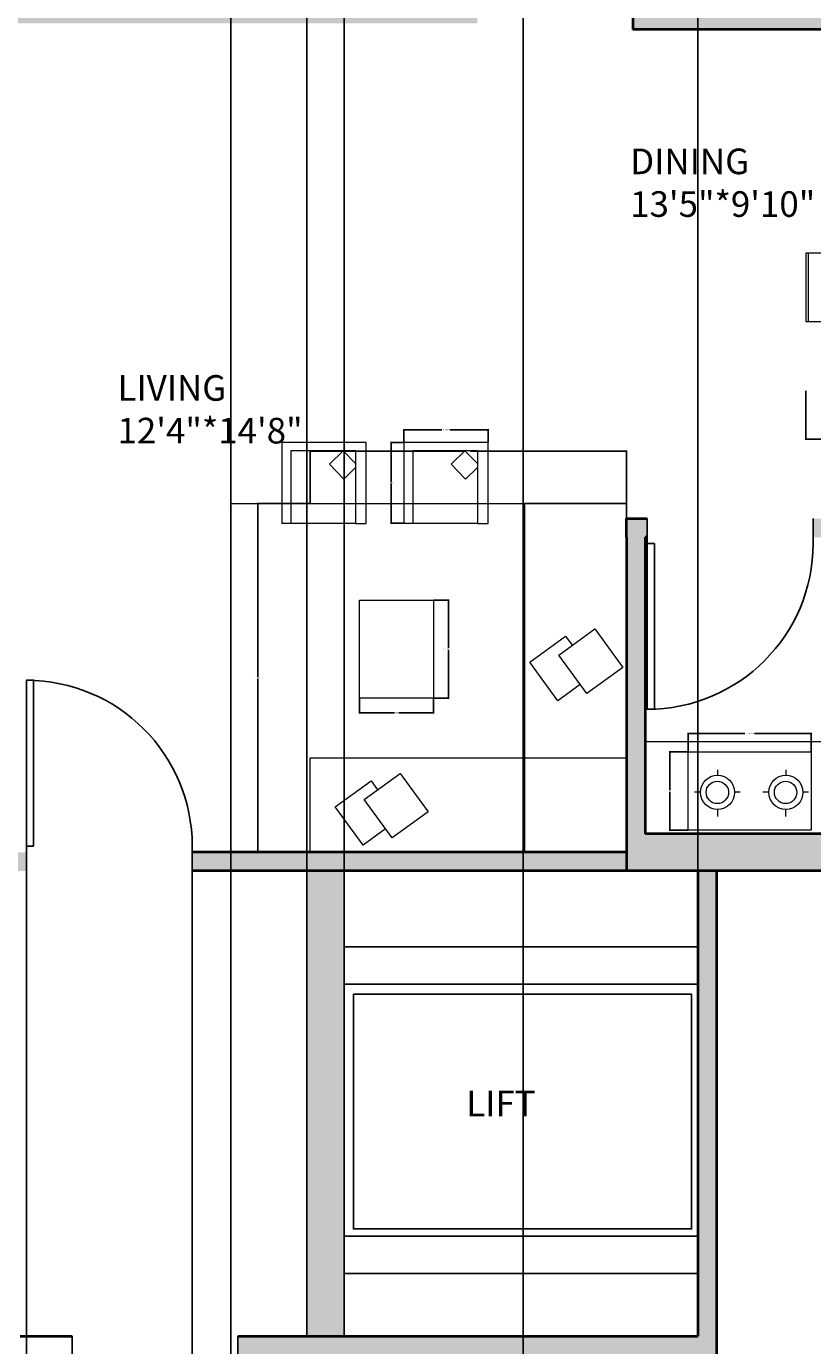
# Model space of a CAD drawing. Units: inches. Extents: x 1642 to 2399, y 1011 to 2291.
# Tile 5 of 7: x 2020 to 2210, y 1595 to 1913. Entities that reach past the tile are written whole.
import ezdxf

# ---------------------------------------------------------------- set-up
doc = ezdxf.new("R2010")
doc.units = ezdxf.units.IN
for name, color, linetype, lineweight in [('A-ANNO-DIMS', 2, 'Continuous', 18), ('A-AREA-IDEN', 7, 'Continuous', 20), ('A-DOOR', 4, 'Continuous', 25), ('A-EQPM', 8, 'Continuous', 18), ('A-FLOR-CASE', 30, 'Continuous', 18), ('A-FLOR-EVTR', 4, 'Continuous', 25), ('A-FURN', 8, 'Continuous', 18), ('A-WALL-PATT', 40, 'Continuous', 13), ('WALL', 40, 'Continuous', 40)]:
    doc.layers.add(name, color=color, linetype=linetype, lineweight=lineweight)
doc.styles.get("Standard").update_dxf_attribs({"font": 'arial.ttf'})
doc.dimstyles.get("Standard").update_dxf_attribs({"dimtxt": 0.18, "dimasz": 0.18, "dimexe": 0.18, "dimexo": 0.0625, "dimgap": 0.09, "dimtad": 0, "dimtih": 1, "dimtoh": 1, "dimdec": 4, "dimzin": 0, "dimdsep": 46, "dimtxsty": 'Standard', "dimcen": 0.09, "dimadec": 0, "dimazin": 0, "dimtfac": 1, "dimtdec": 4, "dimtofl": 0, "dimtmove": 0, "dimatfit": 3, "dimfxl": 1, "dimtolj": 1, "dimtzin": 0, "dimarcsym": 0})

# ---------------------------------------------------------------- blocks, each defined once
blk = doc.blocks.new('*U2')
for p, q in [((0, 0), (0, -6)), ((40, 0), (40, -6))]:
    blk.add_line(p, q)
blk.add_lwpolyline([(0, 0), (0, 40), (1.75, 40), (1.75, 0)], close=True)
blk.add_arc((0, 0), 40, 0, 90)
blk = doc.blocks.new('TABLE-DINING-SIX-SEAT')
for p, q in [((15.31, 48.55), (31.81, 48.55)), ((44.68, 48.55), (61.18, 48.55)), ((0.59, 16.67), (0.59, 33.17)), ((77.22, 16.83), (77.22, 33.33)), ((15.31, 0.59), (31.81, 0.59)), ((44.68, 0.59), (61.18, 0.59))]:
    blk.add_line(p, q)
for points in [[(15.31, 38.77), (31.81, 38.77), (31.81, 49.15), (15.31, 49.15)], [(44.68, 38.77), (61.18, 38.77), (61.18, 49.15), (44.68, 49.15)], [(10.38, 38.77), (67.43, 38.77), (67.43, 10.38), (10.38, 10.38)], [(10.38, 16.67), (10.38, 33.17), (0, 33.17), (0, 16.67)], [(67.43, 16.83), (67.43, 33.33), (77.81, 33.33), (77.81, 16.83)], [(15.31, 10.38), (31.81, 10.38), (31.81, 0), (15.31, 0)], [(44.68, 10.38), (61.18, 10.38), (61.18, 0), (44.68, 0)]]:
    blk.add_lwpolyline(points, close=True)
blk = doc.blocks.new('SEATING-CORNER')
for points in [[(0, 84.13), (76.26, 84.13), (76.26, 61.34), (0, 61.34)], [(0, 0), (24.56, 0), (24.56, 84.13), (0, 84.13)], [(56.51, 80.66), (63.26, 71.39), (54.61, 65.09), (47.86, 74.37)], [(9.57, 45.8), (16.32, 36.53), (7.67, 30.23), (0.92, 39.51)]]:
    blk.add_lwpolyline(points, close=True)
for points in [[(58.1, 78.48), (63.51, 82.42), (70.26, 73.15), (61.61, 66.85), (60.02, 69.03)], [(11.16, 43.62), (16.57, 47.56), (23.32, 38.28), (14.67, 31.99), (13.08, 34.17)]]:
    blk.add_lwpolyline(points)
blk = doc.blocks.new('CHAIR-LOUNGE')
for p, q in [((2.54, 19.51), (0, 19.51)), ((0, 19.51), (0, 0)), ((18.08, 19.51), (20.31, 19.51)), ((20.31, 19.32), (20.31, 19.51)), ((20.31, 0), (20.31, 19.32)), ((0, 0), (20.31, 0))]:
    blk.add_line(p, q)
blk.add_lwpolyline([(2.54, 19.51), (18.08, 19.51), (18.08, 1.93), (2.54, 1.93)], close=True)
blk.add_lwpolyline([(2.54, 6.05), (5.4, 8.82), (8.88, 5.23), (5.55, 2), (2.54, 5.1)])
blk = doc.blocks.new('COOKTOP-TWO-BURNER')
for p, q in [((6.17, 13.89), (6.17, 15.59)), ((22.64, 13.89), (22.64, 15.59)), ((2, 9.67), (0.69, 9.67)), ((10.24, 9.72), (11.69, 9.72)), ((18.47, 9.67), (17.17, 9.67)), ((26.71, 9.72), (28.17, 9.72)), ((6.02, 5.65), (6.02, 4.35)), ((22.49, 5.65), (22.49, 4.35))]:
    blk.add_line(p, q)
blk.add_lwpolyline([(0, 18.89), (29.66, 18.89), (29.66, 0), (0, 0)], close=True)
for centre, radius in [((6.12, 9.77), 4.12), ((22.59, 9.77), 4.12), ((6.17, 9.77), 2.71), ((22.64, 9.77), 2.71)]:
    blk.add_circle(centre, radius)
blk = doc.blocks.new('TABLE-COFFEE')
blk.add_lwpolyline([(0, 23.65), (17.89, 23.65), (17.89, 0), (0, 0)], close=True)
blk = doc.blocks.new('*D16')
at = {"layer": 'A-ANNO-DIMS', "color": 0, "lineweight": -2, "transparency": 16777216}
for p, q in [((2111.47, 1812.9), (2111.47, 1816.06)), ((2111.65, 1815.88), (2120.67, 1815.88)), ((2131.6, 1815.88), (2122.58, 1815.88)), ((2131.78, 1812.9), (2131.78, 1816.06))]:
    blk.add_line(p, q, dxfattribs=at)
at = {"layer": 'A-ANNO-DIMS', "color": 0, "transparency": 16777216}
for points in [[(2111.65, 1815.91), (2111.65, 1815.85), (2111.47, 1815.88)], [(2131.6, 1815.91), (2131.6, 1815.85), (2131.78, 1815.88)]]:
    blk.add_solid(points, dxfattribs=at)
at = {"layer": 'Defpoints', "color": 0, "transparency": 16777216}
for p in [(2111.47, 1815.88), (2111.47, 1812.83), (2131.78, 1812.83)]:
    blk.add_point(p, dxfattribs=at)
at = {"layer": 'A-ANNO-DIMS', "color": 0, "transparency": 16777216, "insert": (2121.63, 1815.88), "char_height": 0.18, "attachment_point": 5}
blk.add_mtext('\\A1;CHAIR 20 TYP.', dxfattribs=at)
blk = doc.blocks.new('*D17')
at = {"layer": 'A-ANNO-DIMS', "color": 0, "lineweight": -2, "transparency": 16777216}
for p, q in [((2111.41, 1812.83), (2108.25, 1812.83)), ((2108.43, 1812.65), (2108.43, 1803.26)), ((2108.43, 1793.51), (2108.43, 1802.9)), ((2111.41, 1793.33), (2108.25, 1793.33))]:
    blk.add_line(p, q, dxfattribs=at)
at = {"layer": 'A-ANNO-DIMS', "color": 0, "transparency": 16777216}
for points in [[(2108.4, 1812.65), (2108.46, 1812.65), (2108.43, 1812.83)], [(2108.4, 1793.51), (2108.46, 1793.51), (2108.43, 1793.33)]]:
    blk.add_solid(points, dxfattribs=at)
at = {"layer": 'Defpoints', "color": 0, "transparency": 16777216}
for p in [(2111.47, 1812.83), (2108.43, 1793.33), (2111.47, 1793.33)]:
    blk.add_point(p, dxfattribs=at)
at = {"layer": 'A-ANNO-DIMS', "color": 0, "transparency": 16777216, "insert": (2108.43, 1803.08), "char_height": 0.18, "attachment_point": 5}
blk.add_mtext('\\A1;20 TYP.', dxfattribs=at)
blk = doc.blocks.new('*D18')
at = {"layer": 'A-ANNO-DIMS', "color": 0, "lineweight": -2, "transparency": 16777216}
for p, q in [((2208.46, 1825.25), (2208.46, 1813.46)), ((2286.28, 1825.25), (2286.28, 1813.46)), ((2208.64, 1813.64), (2246.09, 1813.64)), ((2286.1, 1813.64), (2248.65, 1813.64))]:
    blk.add_line(p, q, dxfattribs=at)
at = {"layer": 'A-ANNO-DIMS', "color": 0, "transparency": 16777216}
for points in [[(2208.64, 1813.67), (2208.64, 1813.61), (2208.46, 1813.64)], [(2286.1, 1813.67), (2286.1, 1813.61), (2286.28, 1813.64)]]:
    blk.add_solid(points, dxfattribs=at)
at = {"layer": 'Defpoints', "color": 0, "transparency": 16777216}
for p in [(2208.46, 1825.31), (2286.28, 1825.31), (2286.28, 1813.64)]:
    blk.add_point(p, dxfattribs=at)
at = {"layer": 'A-ANNO-DIMS', "color": 0, "transparency": 16777216, "insert": (2247.37, 1813.64), "char_height": 0.18, "attachment_point": 5}
blk.add_mtext('\\A1;DINING SET 78 TYP.', dxfattribs=at)
blk = doc.blocks.new('*D20')
at = {"layer": 'A-ANNO-DIMS', "color": 0, "lineweight": -2, "transparency": 16777216}
for p, q in [((2088.86, 1798.08), (2076.12, 1798.08)), ((2076.3, 1797.9), (2076.3, 1756.2)), ((2076.3, 1714.14), (2076.3, 1755.84)), ((2088.86, 1713.96), (2076.12, 1713.96))]:
    blk.add_line(p, q, dxfattribs=at)
at = {"layer": 'A-ANNO-DIMS', "color": 0, "transparency": 16777216}
for points in [[(2076.27, 1797.9), (2076.33, 1797.9), (2076.3, 1798.08)], [(2076.27, 1714.14), (2076.33, 1714.14), (2076.3, 1713.96)]]:
    blk.add_solid(points, dxfattribs=at)
at = {"layer": 'Defpoints', "color": 0, "transparency": 16777216}
for p in [(2088.92, 1798.08), (2076.3, 1713.96), (2088.92, 1713.96)]:
    blk.add_point(p, dxfattribs=at)
at = {"layer": 'A-ANNO-DIMS', "color": 0, "transparency": 16777216, "insert": (2076.3, 1756.02), "char_height": 0.18, "attachment_point": 5}
blk.add_mtext('\\A1;CORNER SOFA 84 TYP.', dxfattribs=at)
blk = doc.blocks.new('*D21')
at = {"layer": 'A-ANNO-DIMS', "color": 0, "lineweight": -2, "transparency": 16777216}
for p, q in [((2088.92, 1798.15), (2088.92, 1810.88)), ((2165.18, 1798.15), (2165.18, 1810.88)), ((2089.1, 1810.7), (2126.52, 1810.7)), ((2165, 1810.7), (2127.58, 1810.7))]:
    blk.add_line(p, q, dxfattribs=at)
at = {"layer": 'A-ANNO-DIMS', "color": 0, "transparency": 16777216}
for points in [[(2089.1, 1810.73), (2089.1, 1810.67), (2088.92, 1810.7)], [(2165, 1810.73), (2165, 1810.67), (2165.18, 1810.7)]]:
    blk.add_solid(points, dxfattribs=at)
at = {"layer": 'Defpoints', "color": 0, "transparency": 16777216}
for p in [(2088.92, 1810.7), (2088.92, 1798.08), (2165.18, 1798.08)]:
    blk.add_point(p, dxfattribs=at)
at = {"layer": 'A-ANNO-DIMS', "color": 0, "transparency": 16777216, "insert": (2127.05, 1810.7), "char_height": 0.18, "attachment_point": 5}
blk.add_mtext('\\A1;76 TYP.', dxfattribs=at)
blk = doc.blocks.new('*D22')
at = {"layer": 'A-ANNO-DIMS', "color": 0, "lineweight": -2, "transparency": 16777216}
for p, q in [((2180.07, 1738.26), (2180.07, 1742.82)), ((2180.25, 1742.64), (2193.71, 1742.64)), ((2209.55, 1742.64), (2196.09, 1742.64)), ((2209.73, 1738.26), (2209.73, 1742.82))]:
    blk.add_line(p, q, dxfattribs=at)
at = {"layer": 'A-ANNO-DIMS', "color": 0, "transparency": 16777216}
for points in [[(2180.25, 1742.67), (2180.25, 1742.61), (2180.07, 1742.64)], [(2209.55, 1742.67), (2209.55, 1742.61), (2209.73, 1742.64)]]:
    blk.add_solid(points, dxfattribs=at)
at = {"layer": 'Defpoints', "color": 0, "transparency": 16777216}
for p in [(2180.07, 1742.64), (2180.07, 1738.19), (2209.73, 1738.19)]:
    blk.add_point(p, dxfattribs=at)
at = {"layer": 'A-ANNO-DIMS', "color": 0, "transparency": 16777216, "insert": (2194.9, 1742.64), "char_height": 0.18, "attachment_point": 5}
blk.add_mtext('\\A1;COOKTOP 30 TYP.', dxfattribs=at)
blk = doc.blocks.new('*D23')
at = {"layer": 'A-ANNO-DIMS', "color": 0, "lineweight": -2, "transparency": 16777216}
for p, q in [((2180.01, 1738.19), (2175.44, 1738.19)), ((2175.62, 1738.01), (2175.62, 1728.93)), ((2175.62, 1719.49), (2175.62, 1728.57)), ((2180.01, 1719.31), (2175.44, 1719.31))]:
    blk.add_line(p, q, dxfattribs=at)
at = {"layer": 'A-ANNO-DIMS', "color": 0, "transparency": 16777216}
for points in [[(2175.59, 1738.01), (2175.65, 1738.01), (2175.62, 1738.19)], [(2175.59, 1719.49), (2175.65, 1719.49), (2175.62, 1719.31)]]:
    blk.add_solid(points, dxfattribs=at)
at = {"layer": 'Defpoints', "color": 0, "transparency": 16777216}
for p in [(2180.07, 1738.19), (2175.62, 1719.31), (2180.07, 1719.31)]:
    blk.add_point(p, dxfattribs=at)
at = {"layer": 'A-ANNO-DIMS', "color": 0, "transparency": 16777216, "insert": (2175.62, 1728.75), "char_height": 0.18, "attachment_point": 5}
blk.add_mtext('\\A1;19 TYP.', dxfattribs=at)
blk = doc.blocks.new('*D28')
at = {"layer": 'A-ANNO-DIMS', "color": 0, "lineweight": -2, "transparency": 16777216}
for p, q in [((2118.74, 1774.81), (2122.4, 1774.81)), ((2122.22, 1774.63), (2122.22, 1763.17)), ((2122.22, 1751.34), (2122.22, 1762.8)), ((2118.74, 1751.16), (2122.4, 1751.16))]:
    blk.add_line(p, q, dxfattribs=at)
at = {"layer": 'A-ANNO-DIMS', "color": 0, "transparency": 16777216}
for points in [[(2122.19, 1774.63), (2122.25, 1774.63), (2122.22, 1774.81)], [(2122.19, 1751.34), (2122.25, 1751.34), (2122.22, 1751.16)]]:
    blk.add_solid(points, dxfattribs=at)
at = {"layer": 'Defpoints', "color": 0, "transparency": 16777216}
for p in [(2118.67, 1774.81), (2118.67, 1751.16), (2122.22, 1751.16)]:
    blk.add_point(p, dxfattribs=at)
at = {"layer": 'A-ANNO-DIMS', "color": 0, "transparency": 16777216, "insert": (2122.22, 1762.99), "char_height": 0.18, "attachment_point": 5}
blk.add_mtext('\\A1;COFFEE TABLE 24 TYP.', dxfattribs=at)
blk = doc.blocks.new('*D29')
at = {"layer": 'A-ANNO-DIMS', "color": 0, "lineweight": -2, "transparency": 16777216}
for p, q in [((2100.78, 1751.1), (2100.78, 1747.43)), ((2118.67, 1751.1), (2118.67, 1747.43)), ((2100.96, 1747.61), (2109.21, 1747.61)), ((2118.49, 1747.61), (2110.25, 1747.61))]:
    blk.add_line(p, q, dxfattribs=at)
at = {"layer": 'A-ANNO-DIMS', "color": 0, "transparency": 16777216}
for points in [[(2100.96, 1747.64), (2100.96, 1747.58), (2100.78, 1747.61)], [(2118.49, 1747.64), (2118.49, 1747.58), (2118.67, 1747.61)]]:
    blk.add_solid(points, dxfattribs=at)
at = {"layer": 'Defpoints', "color": 0, "transparency": 16777216}
for p in [(2100.78, 1751.16), (2118.67, 1751.16), (2100.78, 1747.61)]:
    blk.add_point(p, dxfattribs=at)
at = {"layer": 'A-ANNO-DIMS', "color": 0, "transparency": 16777216, "insert": (2109.73, 1747.61), "char_height": 0.18, "attachment_point": 5}
blk.add_mtext('\\A1;18 TYP.', dxfattribs=at)
blk = doc.blocks.new('*D40')
at = {"layer": 'A-ANNO-DIMS', "color": 0, "lineweight": -2, "transparency": 16777216}
for p, q in [((1796.18, 1709.39), (1796.18, 1011.19)), ((2186.88, 1709.39), (2186.88, 1011.19)), ((1796.36, 1011.37), (1991.13, 1011.37)), ((2186.7, 1011.37), (1991.92, 1011.37))]:
    blk.add_line(p, q, dxfattribs=at)
at = {"layer": 'A-ANNO-DIMS', "color": 0, "transparency": 16777216}
for points in [[(1796.36, 1011.4), (1796.36, 1011.34), (1796.18, 1011.37)], [(2186.7, 1011.4), (2186.7, 1011.34), (2186.88, 1011.37)]]:
    blk.add_solid(points, dxfattribs=at)
at = {"layer": 'Defpoints', "color": 0, "transparency": 16777216}
for p in [(1796.18, 1709.46), (2186.88, 1709.46), (2186.88, 1011.37)]:
    blk.add_point(p, dxfattribs=at)
at = {"layer": 'A-ANNO-DIMS', "color": 0, "transparency": 16777216, "insert": (1991.53, 1011.37), "char_height": 0.18, "attachment_point": 5}
blk.add_mtext('\\A1;390.7', dxfattribs=at)
blk = doc.blocks.new('*D42')
at = {"layer": 'A-ANNO-DIMS', "color": 0, "lineweight": -2, "transparency": 16777216}
for p, q in [((1946.68, 1597.27), (1946.68, 2290.98)), ((1946.86, 2290.8), (2016.99, 2290.8)), ((2087.89, 2290.8), (2017.76, 2290.8)), ((2088.07, 1597.27), (2088.07, 2290.98))]:
    blk.add_line(p, q, dxfattribs=at)
at = {"layer": 'A-ANNO-DIMS', "color": 0, "transparency": 16777216}
for points in [[(1946.86, 2290.83), (1946.86, 2290.77), (1946.68, 2290.8)], [(2087.89, 2290.83), (2087.89, 2290.77), (2088.07, 2290.8)]]:
    blk.add_solid(points, dxfattribs=at)
at = {"layer": 'Defpoints', "color": 0, "transparency": 16777216}
for p in [(2088.07, 2290.8), (1946.68, 1597.21), (2088.07, 1597.21)]:
    blk.add_point(p, dxfattribs=at)
at = {"layer": 'A-ANNO-DIMS', "color": 0, "transparency": 16777216, "insert": (2017.37, 2290.8), "char_height": 0.18, "attachment_point": 5}
blk.add_mtext('\\A1;141.4', dxfattribs=at)
blk = doc.blocks.new('*D43')
at = {"layer": 'A-ANNO-DIMS', "color": 0, "lineweight": -2, "transparency": 16777216}
for p, q in [((2097.07, 1597.27), (2097.07, 2290.98)), ((2097.25, 2290.8), (2139.35, 2290.8)), ((2182.2, 2290.8), (2140.1, 2290.8)), ((2182.38, 1597.27), (2182.38, 2290.98))]:
    blk.add_line(p, q, dxfattribs=at)
at = {"layer": 'A-ANNO-DIMS', "color": 0, "transparency": 16777216}
for points in [[(2097.25, 2290.83), (2097.25, 2290.77), (2097.07, 2290.8)], [(2182.2, 2290.83), (2182.2, 2290.77), (2182.38, 2290.8)]]:
    blk.add_solid(points, dxfattribs=at)
at = {"layer": 'Defpoints', "color": 0, "transparency": 16777216}
for p in [(2182.38, 2290.8), (2097.07, 1597.21), (2182.38, 1597.21)]:
    blk.add_point(p, dxfattribs=at)
at = {"layer": 'A-ANNO-DIMS', "color": 0, "transparency": 16777216, "insert": (2139.72, 2290.8), "char_height": 0.18, "attachment_point": 5}
blk.add_mtext('\\A1;85.31', dxfattribs=at)
blk = doc.blocks.new('*D46')
at = {"layer": 'A-ANNO-DIMS', "color": 0, "lineweight": -2, "transparency": 16777216}
for p, q in [((2020.45, 1709.39), (2020.45, 1011.19)), ((2060.45, 1709.39), (2060.45, 1011.19)), ((2020.63, 1011.37), (2040.22, 1011.37)), ((2060.27, 1011.37), (2040.67, 1011.37))]:
    blk.add_line(p, q, dxfattribs=at)
at = {"layer": 'A-ANNO-DIMS', "color": 0, "transparency": 16777216}
for points in [[(2020.63, 1011.4), (2020.63, 1011.34), (2020.45, 1011.37)], [(2060.27, 1011.4), (2060.27, 1011.34), (2060.45, 1011.37)]]:
    blk.add_solid(points, dxfattribs=at)
at = {"layer": 'Defpoints', "color": 0, "transparency": 16777216}
for p in [(2020.45, 1709.46), (2060.45, 1709.46), (2060.45, 1011.37)]:
    blk.add_point(p, dxfattribs=at)
at = {"layer": 'A-ANNO-DIMS', "color": 0, "transparency": 16777216, "insert": (2040.45, 1011.37), "char_height": 0.18, "attachment_point": 5}
blk.add_mtext('\\A1;40', dxfattribs=at)
blk = doc.blocks.new('*D48')
at = {"layer": 'A-ANNO-DIMS', "color": 0, "lineweight": -2, "transparency": 16777216}
for p, q in [((1922.74, 1392.77), (1922.74, 2290.98)), ((1922.92, 2290.8), (2031.1, 2290.8)), ((2140.06, 2290.8), (2031.89, 2290.8)), ((2140.24, 1392.77), (2140.24, 2290.98))]:
    blk.add_line(p, q, dxfattribs=at)
at = {"layer": 'A-ANNO-DIMS', "color": 0, "transparency": 16777216}
for points in [[(1922.92, 2290.83), (1922.92, 2290.77), (1922.74, 2290.8)], [(2140.06, 2290.83), (2140.06, 2290.77), (2140.24, 2290.8)]]:
    blk.add_solid(points, dxfattribs=at)
at = {"layer": 'Defpoints', "color": 0, "transparency": 16777216}
for p in [(2140.24, 2290.8), (1922.74, 1392.71), (2140.24, 1392.71)]:
    blk.add_point(p, dxfattribs=at)
at = {"layer": 'A-ANNO-DIMS', "color": 0, "transparency": 16777216, "insert": (2031.49, 2290.8), "char_height": 0.18, "attachment_point": 5}
blk.add_mtext('\\A1;217.5', dxfattribs=at)
blk = doc.blocks.new('*D50')
at = {"layer": 'A-ANNO-DIMS', "color": 0, "lineweight": -2, "transparency": 16777216}
for p, q in [((1993.24, 1295.77), (1993.24, 2290.98)), ((1993.42, 2290.8), (2031.17, 2290.8)), ((2069.56, 2290.8), (2031.82, 2290.8)), ((2069.74, 1295.77), (2069.74, 2290.98))]:
    blk.add_line(p, q, dxfattribs=at)
at = {"layer": 'A-ANNO-DIMS', "color": 0, "transparency": 16777216}
for points in [[(1993.42, 2290.83), (1993.42, 2290.77), (1993.24, 2290.8)], [(2069.56, 2290.83), (2069.56, 2290.77), (2069.74, 2290.8)]]:
    blk.add_solid(points, dxfattribs=at)
at = {"layer": 'Defpoints', "color": 0, "transparency": 16777216}
for p in [(2069.74, 2290.8), (1993.24, 1295.71), (2069.74, 1295.71)]:
    blk.add_point(p, dxfattribs=at)
at = {"layer": 'A-ANNO-DIMS', "color": 0, "transparency": 16777216, "insert": (2031.49, 2290.8), "char_height": 0.18, "attachment_point": 5}
blk.add_mtext('\\A1;76.5', dxfattribs=at)

msp = doc.modelspace()

# ---------------------------------------------------------------- hatches: boundary and pattern name
at = {"layer": 'A-WALL-PATT'}
h = msp.add_hatch(color=256, dxfattribs=at)
h.dxf.hatch_style = 1
h.paths.add_polyline_path([(2340.1804, 2185.4562), (2211.0983, 2185.4562, -0.01876983), (2211.211, 2182.4562), (2211.211, 2176.4562), (2331.211, 2176.4562), (2331.211, 2043.4562), (2171.211, 2043.4562), (2171.211, 2038.9562), (2331.211, 2038.9562), (2331.211, 1916.9562), (2171.211, 1916.9562), (2171.211, 1918.9365), (2166.711, 1918.9365), (2166.711, 1912.4562), (2340.1804, 1912.4562)])
h.paths.add_polyline_path([(2171.211, 2043.4562), (2171.211, 2043.9025), (2170.5217, 2043.9025), (2166.711, 2043.9025), (2166.711, 2038.9562), (2166.711, 1958.9365), (2171.211, 1958.9365)], flags=17)
h.paths.add_polyline_path([(2129.211, 1971.5979), (2124.711, 1971.5979), (2124.711, 1918.4562), (2067.711, 1918.4562), (2067.711, 1913.9562), (2129.211, 1913.9562)])
h.paths.add_polyline_path([(2067.711, 2015.4562), (2124.711, 2015.4562), (2124.711, 2019.9562), (2058.711, 2019.9562), (2058.711, 2015.4562), (2058.711, 1922.9562), (1982.211, 1922.9562), (1982.211, 2015.4562), (1982.211, 2019.9562), (1916.211, 2019.9562), (1916.211, 2070.9562), (1911.711, 2070.9562), (1911.711, 2015.4562), (1911.711, 2012.302), (1916.211, 2012.302), (1916.211, 2015.4562), (1973.211, 2015.4562), (1973.211, 1918.4562), (1973.211, 1913.9562), (2017.1804, 1913.9562), (2067.711, 1913.9562), (2067.711, 1918.4562)])
h.paths.add_polyline_path([(2131.1386, 2075.4562), (2118.1934, 2075.4562), (2118.1934, 2070.9562), (2131.1386, 2070.9562)], flags=17)
h.paths.add_polyline_path([(1918.8034, 2075.4562), (1909.4956, 2075.4562), (1909.4956, 2070.9562), (1918.8034, 2070.9562)], flags=17)
h.paths.add_polyline_path([(1874.211, 2029.9562), (1869.711, 2029.9562), (1869.711, 1960.7404), (1874.211, 1960.7404)], flags=17)
h.paths.add_polyline_path([(1916.211, 1972.302), (1911.711, 1972.302), (1911.711, 1918.4562), (1916.211, 1918.4562)], flags=17)
h.paths.add_polyline_path([(2340.1804, 1912.4562), (2331.1804, 1912.4562), (2331.1804, 1794.4562), (2210.1804, 1794.4562), (2210.1804, 1789.9562), (2279.6804, 1789.9562), (2340.1804, 1789.9562)])
h.paths.add_polyline_path([(2288.6804, 1789.9562), (2279.6804, 1789.9562), (2279.6804, 1785.0846), (2285.6804, 1785.0846), (2288.6804, 1785.0846)], flags=17)
h.paths.add_polyline_path([(2169.6804, 1789.9562), (2170.1804, 1789.9562), (2170.1804, 1794.4562), (2165.1804, 1794.4562), (2165.1804, 1713.9562), (2165.1804, 1709.4562), (2279.6804, 1709.4562), (2279.6804, 1718.4562), (2169.6804, 1718.4562)])
h.paths.add_polyline_path([(2288.6804, 1745.1973, -0.01876983), (2285.6804, 1745.0846), (2279.6804, 1745.0846), (2279.6804, 1709.4562), (2340.1804, 1709.4562), (2340.1804, 1789.9562), (2335.6804, 1789.9562), (2335.6804, 1713.9562), (2288.6804, 1713.9562)])
h.paths.add_polyline_path([(2165.1804, 1713.9562), (2140.6229, 1713.9562), (2088.923, 1713.9562), (2069.7509, 1713.9562), (2060.4457, 1713.9562), (2060.4457, 1709.4562), (2165.1804, 1709.4562)])
h.paths.add_polyline_path([(2020.4457, 1713.9562), (2017.1804, 1713.9562), (2012.6804, 1713.9562), (2009.1946, 1713.9562), (2009.1946, 1709.4562), (2020.4457, 1709.4562)])
h.paths.add_polyline_path([(1969.1946, 1713.9562), (1864.6804, 1713.9562), (1864.6804, 1798.9562), (1860.1804, 1798.9562), (1860.1804, 1792.9562), (1860.1804, 1752.9562), (1860.1804, 1718.4562), (1750.1804, 1718.4562), (1750.1804, 1749.2419), (1744.1804, 1749.2419, -0.01876983), (1741.1804, 1749.3546), (1741.1804, 1709.4562), (1969.1946, 1709.4562)])
h.paths.add_polyline_path([(1741.1804, 1803.4562), (1700.711, 1803.4562), (1700.711, 1794.4562), (1741.1804, 1794.4562)])
h.paths.add_polyline_path([(1820.1804, 1798.9562), (1741.1804, 1798.9562), (1741.1804, 1794.4562), (1741.1804, 1790.0365), (1741.1804, 1789.2419), (1744.1804, 1789.2419), (1750.1804, 1789.2419), (1750.1804, 1794.4562), (1820.1804, 1794.4562)], flags=17)
h.paths.add_polyline_path([(1800.6804, 1709.4562), (1796.1804, 1709.4562), (1796.1804, 1592.7078), (1978.9325, 1592.7078), (1978.9325, 1597.2078), (1800.6804, 1597.2078)])
h.paths.add_polyline_path([(2097.0678, 1709.4562), (2088.0678, 1709.4562), (2088.0678, 1599.6874), (2088.0678, 1597.2078), (2097.0678, 1597.2078)], flags=17)
h.paths.add_polyline_path([(2186.8766, 1709.4562), (2182.3766, 1709.4562), (2182.3766, 1597.2078), (2071.4624, 1597.2078), (2071.4624, 1592.7078), (2186.8766, 1592.7078)])
h.paths.add_polyline_path([(2078.1934, 2075.4562), (2022.711, 2075.4562), (2022.711, 2223.4562), (2166.711, 2223.4562), (2166.711, 2075.4562), (2166.711, 2070.9562), (2171.211, 2070.9562), (2171.211, 2138.8919), (2171.211, 2227.9562), (2335.711, 2227.9562), (2335.711, 2185.4562), (2340.1804, 2185.4562), (2340.1804, 2232.4562), (1874.211, 2232.4562), (1874.211, 2223.4562), (2018.211, 2223.4562), (2018.211, 2075.4562), (1958.8034, 2075.4562), (1958.8034, 2070.9562), (2018.211, 2070.9562), (2018.211, 2019.9562), (1982.211, 2019.9562), (1982.211, 2015.4562), (1982.211, 2010.9562), (2058.711, 2010.9562), (2058.711, 2015.4562), (2058.711, 2019.9562), (2022.711, 2019.9562), (2022.711, 2070.9562), (2078.1934, 2070.9562)])
h.paths.add_polyline_path([(1874.211, 2171.9562), (1874.211, 2176.4562), (1861.9371, 2176.4562), (1861.9371, 2173.4562), (1861.9371, 2167.4562), (1869.711, 2167.4562), (1869.711, 2069.7602), (1874.211, 2069.7602)], flags=17)
h.paths.add_polyline_path([(1705.211, 2227.9562), (1865.211, 2227.9562), (1865.211, 2176.4562), (1874.211, 2176.4562), (1874.211, 2232.4562), (1700.711, 2232.4562), (1700.711, 2176.4562), (1705.211, 2176.4562)])
h.paths.add_polyline_path([(1709.711, 2167.4562), (1821.9371, 2167.4562), (1821.9371, 2173.4562, -0.01876983), (1822.0498, 2176.4562), (1700.711, 2176.4562), (1700.711, 1913.9562), (1860.1804, 1913.9562), (1864.6804, 1913.9562), (1973.211, 1913.9562), (1973.211, 1918.4562), (1916.211, 1918.4562), (1874.211, 1918.4562), (1874.211, 1920.7404), (1869.711, 1920.7404), (1869.711, 1918.4562), (1860.1804, 1918.4562), (1709.711, 1918.4562), (1709.711, 2029.9562), (1874.211, 2029.9562), (1874.211, 2037.0364), (1869.711, 2037.0364), (1869.711, 2034.4562), (1709.711, 2034.4562)])
h.paths.add_polyline_path([(2017.1804, 1913.9562), (2012.6804, 1913.9562), (2012.6804, 1713.9562), (2017.1804, 1713.9562)])
h.paths.add_polyline_path([(1952.4341, 2110.3716), (2000.4134, 2110.3716), (2000.4134, 2133.4189), (1952.4341, 2133.4189)], flags=25)
h.paths.add_polyline_path([(2042.3983, 2110.7121), (2090.3775, 2110.7121), (2090.3775, 2133.7594), (2042.3983, 2133.7594)], flags=25)
h.paths.add_polyline_path([(2201.7332, 2091.8715), (2249.7125, 2091.8715), (2249.7125, 2114.9188), (2201.7332, 2114.9188)], flags=25)
h.paths.add_polyline_path([(1805.186, 2077.6915), (1853.1653, 2077.6915), (1853.1653, 2100.7388), (1805.186, 2100.7388)], flags=25)
h.paths.add_polyline_path([(1794.8897, 1974.6584), (1842.869, 1974.6584), (1842.869, 1997.7057), (1794.8897, 1997.7057)], flags=25)
h.paths.add_polyline_path([(2229.1796, 2204.4209), (2315.1362, 2204.4209), (2315.1362, 2217.1488), (2229.1796, 2217.1488)], flags=25)
h.paths.add_polyline_path([(1715.2159, 2199.5328), (1801.1724, 2199.5328), (1801.1724, 2212.2607), (1715.2159, 2212.2607)], flags=25)
h.paths.add_polyline_path([(2230.7681, 1755.7109), (2271.7283, 1755.7109), (2271.7283, 1778.7582), (2230.7681, 1778.7582)], flags=25)
h.paths.add_polyline_path([(1763.4713, 1764.1742), (1804.4315, 1764.1742), (1804.4315, 1787.2215), (1763.4713, 1787.2215)], flags=25)
h.paths.add_polyline_path([(2076.2643, 1955.0495), (2111.326, 1955.0495), (2111.326, 1978.0968), (2076.2643, 1978.0968)], flags=25)
h.paths.add_polyline_path([(1932.854, 1956.1217), (1967.9158, 1956.1217), (1967.9158, 1979.169), (1932.854, 1979.169)], flags=25)
h.paths.add_polyline_path([(2048.1203, 2031.6107), (2083.1821, 2031.6107), (2083.1821, 2054.658), (2048.1203, 2054.658)], flags=25)
h.paths.add_polyline_path([(2163.5754, 1863.7569), (2208.2347, 1863.7569), (2208.2347, 1886.8042), (2163.5754, 1886.8042)], flags=9)
h.paths.add_polyline_path([(2039.9286, 1809.0957), (2084.5879, 1809.0957), (2084.5879, 1832.143), (2039.9286, 1832.143)], flags=9)
h.paths.add_polyline_path([(1901.0045, 1814.0452), (1945.6638, 1814.0452), (1945.6638, 1837.0925), (1901.0045, 1837.0925)], flags=9)
h.paths.add_polyline_path([(1833.7282, 1852.5627), (1878.3875, 1852.5627), (1878.3875, 1875.61), (1833.7282, 1875.61)], flags=9)
h.paths.add_polyline_path([(2219.1375, 1926.2139), (2267.1167, 1926.2139), (2267.1167, 1949.2612), (2219.1375, 1949.2612)], flags=25)
h.paths.add_polyline_path([(1956.9598, 2029.7735), (1992.0216, 2029.7735), (1992.0216, 2052.8208), (1956.9598, 2052.8208)], flags=25)
h.paths.add_polyline_path([(2229.3, 1523.3399), (2270.2602, 1523.3399), (2270.2602, 1546.3872), (2229.3, 1546.3872)], flags=9)
h.paths.add_polyline_path([(1772.3039, 1526.9922), (1813.2641, 1526.9922), (1813.2641, 1550.0394), (1772.3039, 1550.0394)], flags=9)
h.paths.add_polyline_path([(2172.587, 1420.6999), (2217.2463, 1420.6999), (2217.2463, 1443.7472), (2172.587, 1443.7472)], flags=9)
h.paths.add_polyline_path([(1814.3549, 1422.215), (1859.0143, 1422.215), (1859.0143, 1445.2623), (1814.3549, 1445.2623)], flags=9)
h.paths.add_polyline_path([(2186.0372, 1305.6227), (2234.0165, 1305.6227), (2234.0165, 1328.67), (2186.0372, 1328.67)], flags=9)
h.paths.add_polyline_path([(1756.747, 1349.0694), (1804.7263, 1349.0694), (1804.7263, 1372.1167), (1756.747, 1372.1167)], flags=9)
h.paths.add_polyline_path([(2239.449, 1214.6184), (2287.4282, 1214.6184), (2287.4282, 1237.6657), (2239.449, 1237.6657)], flags=9)
h.paths.add_polyline_path([(1767.104, 1213.8348), (1815.0832, 1213.8348), (1815.0832, 1236.8821), (1767.104, 1236.8821)], flags=9)
h.paths.add_polyline_path([(2046.6809, 1183.6854), (2094.6602, 1183.6854), (2094.6602, 1206.7327), (2046.6809, 1206.7327)], flags=9)
h.paths.add_polyline_path([(1947.2155, 1183.6854), (1995.1948, 1183.6854), (1995.1948, 1206.7327), (1947.2155, 1206.7327)], flags=9)
h.paths.add_polyline_path([(1959.3556, 1258.7871), (1994.4174, 1258.7871), (1994.4174, 1281.8344), (1959.3556, 1281.8344)], flags=9)
h.paths.add_polyline_path([(2049.6419, 1248.9629), (2084.7036, 1248.9629), (2084.7036, 1272.0102), (2049.6419, 1272.0102)], flags=9)
h.paths.add_polyline_path([(2092.7532, 1327.4852), (2127.815, 1327.4852), (2127.815, 1350.5325), (2092.7532, 1350.5325)], flags=9)
h.paths.add_polyline_path([(1944.9358, 1327.4852), (1979.9976, 1327.4852), (1979.9976, 1350.5325), (1944.9358, 1350.5325)], flags=9)
h.paths.add_polyline_path([(1974.5055, 1650.063), (2006.3695, 1650.063), (2006.3695, 1662.7909), (1974.5055, 1662.7909)], flags=9)

# ---------------------------------------------------------------- linework, layer by layer
at = {"layer": 'A-FLOR-CASE'}
msp.add_line((2279.6804, 1740.5928), (2169.6804, 1740.5928), dxfattribs=at)
at = {"layer": 'A-FLOR-EVTR'}
for p, q in [((2088.0678, 1599.6874), (2088.0678, 1711.9358)), ((2088.0678, 1597.2078), (2088.0678, 1709.4562)), ((2097.0678, 1597.2078), (2097.0678, 1709.4562)), ((2097.0678, 1691.1483), (2182.3766, 1691.1483)), ((2097.0678, 1682.1483), (2182.3766, 1682.1483)), ((2097.0678, 1621.3756), (2182.3766, 1621.3756)), ((2097.0678, 1612.3756), (2182.3766, 1612.3756))]:
    msp.add_line(p, q, dxfattribs=at)
msp.add_lwpolyline([(2099.3395, 1679.7065), (2180.8762, 1679.7065), (2180.8762, 1623.0927), (2099.3395, 1623.0927)], close=True, dxfattribs=at)
at = {"layer": 'A-FURN'}
msp.add_lwpolyline([(2165.1804, 1713.9562), (2069.7509, 1713.9562), (2069.7509, 1798.0844), (2165.1804, 1798.0844)], close=True, dxfattribs=at)
at = {"layer": 'WALL'}
for p, q in [((2166.711, 1918.9365), (2166.711, 1912.4562)), ((2340.211, 1912.4562), (2166.711, 1912.4562)), ((2165.1804, 1789.9562), (2165.1804, 1794.4562)), ((2165.1804, 1794.4562), (2170.1804, 1794.4562)), ((2165.1804, 1789.9562), (2165.1804, 1709.4562)), ((2169.6804, 1789.9562), (2169.6804, 1718.4562)), ((2170.1804, 1789.9562), (2169.6804, 1789.9562)), ((2279.6804, 1718.4562), (2169.6804, 1718.4562)), ((2165.1804, 1713.9562), (2060.4457, 1713.9562)), ((2165.1804, 1713.9562), (2060.4457, 1713.9562)), ((2165.1804, 1709.4562), (2060.4457, 1709.4562)), ((2279.6804, 1709.4562), (2165.1804, 1709.4562)), ((2182.3766, 1709.4562), (2182.3766, 1597.2078)), ((2186.8766, 1709.4562), (2186.8766, 1592.7078)), ((2018.9325, 1597.2078), (2031.4624, 1597.2078)), ((2071.4624, 1597.2078), (2182.3766, 1597.2078))]:
    msp.add_line(p, q, dxfattribs=at)
msp.add_lwpolyline([(1969.1946, 1709.4562), (1700.711, 1709.4562), (1700.711, 2232.4562), (2340.1804, 2232.4562), (2340.1804, 1709.4562), (2060.4457, 1709.4562)], dxfattribs=at)

# ---------------------------------------------------------------- block references
at = {"layer": 'A-DOOR', "xscale": -1, "rotation": 180}
for p in [(2170.1804, 1788.4562), (2031.4624, 1591.2078)]:
    msp.add_blockref('*U2', p, dxfattribs=at)
at = {"layer": 'A-DOOR'}
msp.add_blockref('*U2', (2020.4457, 1715.4562), dxfattribs=at)
at = {"layer": 'A-EQPM', "rotation": 180}
msp.add_blockref('COOKTOP-TWO-BURNER', (2209.7344, 1738.1937), dxfattribs=at)
at = {"layer": 'A-FURN'}
msp.add_blockref('TABLE-DINING-SIX-SEAT', (2208.4629, 1825.31), dxfattribs=at)
at = {"layer": 'A-FURN', "rotation": 180}
for name, p in [('CHAIR-LOUNGE', (2102.3913, 1812.8329)), ('CHAIR-LOUNGE', (2131.78, 1812.8329)), ('SEATING-CORNER', (2165.1804, 1798.0844)), ('TABLE-COFFEE', (2118.6736, 1774.8115))]:
    msp.add_blockref(name, p, dxfattribs=at)

# ---------------------------------------------------------------- texts
at = {"layer": 'A-AREA-IDEN', "attachment_point": 1}
for s, insert, char_height in [('DINING\\P13\'5"*9\'10"', (2166.059, 1883.7307), 6.176468), ('LIVING\\P12\'4"*14\'8"', (2042.4122, 1829.0695), 6.176468), ('LIFT', (2126.529, 1656.4594), 6.17647)]:
    msp.add_mtext_dynamic_manual_height_columns(s, width=136.850471, gutter_width=30.8823, heights=[0], dxfattribs=dict(at, insert=insert, char_height=char_height))

# ---------------------------------------------------------------- dimensions: what is measured, and where the dimension line sits
at = {"layer": 'A-ANNO-DIMS'}
for base, p1, p2, override, picture, middle in [((2140.2415, 2290.7962), (1922.7415, 1392.7078), (2140.2415, 1392.7078), {"dimdec": 1, "dimlfac": 1, "dimrnd": 0, "dimzin": 0, "dimdsep": 46, "dimlunit": 2}, '*D48', (2031.4915, 2290.7962)), ((2088.0678, 2290.7962), (1946.6804, 1597.2078), (2088.0678, 1597.2078), {"dimdec": 1, "dimlfac": 1, "dimrnd": 0, "dimzin": 0, "dimdsep": 46, "dimlunit": 2}, '*D42', (2017.3741, 2290.7962)), ((2069.7415, 2290.7962), (1993.2415, 1295.7078), (2069.7415, 1295.7078), {"dimdec": 1, "dimlfac": 1, "dimrnd": 0, "dimzin": 0, "dimdsep": 46, "dimlunit": 2}, '*D50', (2031.4915, 2290.7962)), ((2182.3766, 2290.7962), (2097.0678, 1597.2078), (2182.3766, 1597.2078), {"dimdec": 2, "dimlfac": 1, "dimrnd": 0, "dimzin": 0, "dimdsep": 46, "dimlunit": 2}, '*D43', (2139.7222, 2290.7962)), ((2186.8766, 1011.3678), (1796.1804, 1709.4562), (2186.8766, 1709.4562), {"dimdec": 1, "dimlfac": 1, "dimrnd": 0, "dimzin": 0, "dimdsep": 46, "dimlunit": 2}, '*D40', (1991.5285, 1011.3678)), ((2060.4457, 1011.3678), (2020.4457, 1709.4562), (2060.4457, 1709.4562), {"dimdec": 0, "dimlfac": 1, "dimrnd": 0, "dimzin": 0, "dimdsep": 46, "dimlunit": 2}, '*D46', (2040.4457, 1011.3678))]:
    dim = msp.add_linear_dim(base=base, p1=p1, p2=p2, dimstyle='Standard', override=override, dxfattribs=at)
    dim.commit()
    dim.dimension.update_dxf_attribs({"geometry": picture, "text_midpoint": middle})
dim = msp.add_linear_dim(base=(2286.2767, 1813.6379), p1=(2208.4629, 1825.31), p2=(2286.2767, 1825.31), text='DINING SET <> TYP.', dimstyle='Standard', override={"dimdec": 0, "dimlfac": 1, "dimrnd": 0, "dimzin": 0, "dimdsep": 46, "dimlunit": 2}, dxfattribs=at)
dim.commit()
dim.dimension.update_dxf_attribs({"geometry": '*D18', "text_midpoint": (2247.3698, 1813.6379)})
for base, p1, p2, angle, text, picture, middle in [((2111.4716, 1815.8792), (2131.78, 1812.8329), (2111.4716, 1812.8329), 180, 'CHAIR <> TYP.', '*D16', (2121.6258, 1815.8792)), ((2088.923, 1810.7037), (2165.1804, 1798.0844), (2088.923, 1798.0844), 180, '<> TYP.', '*D21', (2127.0517, 1810.7037)), ((2108.4254, 1793.3263), (2111.4716, 1812.8329), (2111.4716, 1793.3263), 270, '<> TYP.', '*D17', (2108.4254, 1803.0796)), ((2076.3037, 1713.9562), (2088.923, 1798.0844), (2088.923, 1713.9562), 270, 'CORNER SOFA <> TYP.', '*D20', (2076.3037, 1756.0203)), ((2122.2214, 1751.1596), (2118.6736, 1774.8115), (2118.6736, 1751.1596), 270, 'COFFEE TABLE <> TYP.', '*D28', (2122.2214, 1762.9856)), ((2100.7818, 1747.6119), (2118.6736, 1751.1596), (2100.7818, 1751.1596), 180, '<> TYP.', '*D29', (2109.7277, 1747.6119)), ((2180.073, 1742.6429), (2209.7344, 1738.1937), (2180.073, 1738.1937), 180, 'COOKTOP <> TYP.', '*D22', (2194.9037, 1742.6429)), ((2175.6238, 1719.3057), (2180.073, 1738.1937), (2180.073, 1719.3057), 270, '<> TYP.', '*D23', (2175.6238, 1728.7497))]:
    dim = msp.add_linear_dim(base=base, p1=p1, p2=p2, angle=angle, text=text, dimstyle='Standard', override={"dimdec": 0, "dimlfac": 1, "dimrnd": 0, "dimzin": 0, "dimdsep": 46, "dimlunit": 2}, dxfattribs=at)
    dim.commit()
    dim.dimension.update_dxf_attribs({"geometry": picture, "text_midpoint": middle})

doc.saveas('drawing.dxf')
